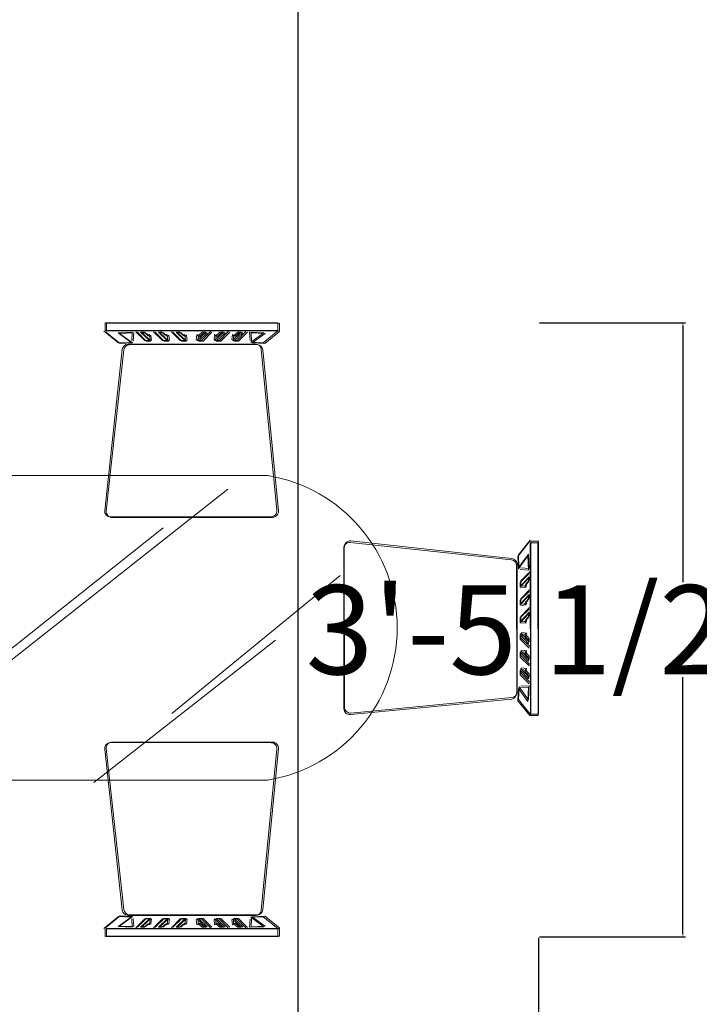
# Model space of a CAD drawing. Units: inches. Extents: x -26 to 575, y -18 to 513.
# Tile 7 of 28: x 77 to 122, y 257 to 324. Entities that reach past the tile are written whole.
import ezdxf

# ---------------------------------------------------------------- set-up
doc = ezdxf.new("R2010")
doc.units = ezdxf.units.IN
doc.header["$MEASUREMENT"] = 0
doc.layers.add('A-ANNO-DIMS', color=2, linetype='Continuous', lineweight=18)
doc.layers.add('Furniture', color=8, linetype='Continuous', lineweight=15)
doc.styles.get("Standard").update_dxf_attribs({"font": 'arial.ttf', "height": 6})
doc.dimstyles.get("Standard").update_dxf_attribs({"dimtxt": 6, "dimasz": 0.18, "dimexe": 0.18, "dimexo": 0.0625, "dimgap": 0.09, "dimtad": 0, "dimtih": 1, "dimtoh": 1, "dimzin": 0, "dimdsep": 46, "dimlunit": 3, "dimtxsty": 'Standard', "dimcen": 0.09, "dimadec": 0, "dimazin": 0, "dimtfac": 1, "dimtofl": 0, "dimtmove": 0, "dimatfit": 3, "dimfxl": 1, "dimtolj": 1, "dimtzin": 0, "dimarcsym": 0})

# ---------------------------------------------------------------- blocks, each defined once
blk = doc.blocks.new('DINING-SET-6-SEAT')
for p, q in [((16.828, 40.76, -3.573), (16.828, 41.278, -3.573)), ((16.828, 41.278, -3.573), (28.461, 41.278, -3.573)), ((16.931, 40.798, -3.573), (16.931, 41.316, -3.573)), ((16.931, 41.316, -3.573), (28.564, 41.316, -3.573)), ((28.461, 41.278, -3.573), (28.461, 40.76, -3.573)), ((28.564, 41.316, -3.573), (28.564, 40.798, -3.573)), ((47.187, 41.329, -3.573), (35.554, 41.319, -3.573)), ((35.554, 41.319, -3.573), (35.554, 40.801, -3.573)), ((47.29, 41.291, -3.573), (35.657, 41.281, -3.573)), ((35.657, 41.281, -3.573), (35.657, 40.763, -3.573)), ((47.188, 40.811, -3.573), (47.187, 41.329, -3.573)), ((47.29, 40.774, -3.573), (47.29, 41.291, -3.573)), ((28.461, 40.76, -3.573), (16.828, 40.76, -3.573)), ((16.828, 40.72, -3.573), (17.824, 39.924, -3.573)), ((28.564, 40.798, -3.573), (16.931, 40.798, -3.573)), ((16.931, 40.758, -3.573), (17.927, 39.962, -3.573)), ((17.784, 40.601, -3.573), (18.74, 40.641, -3.573)), ((18.661, 39.964, -3.573), (17.784, 40.601, -3.573)), ((17.887, 40.639, -3.573), (18.843, 40.679, -3.573)), ((18.763, 40.002, -3.573), (17.887, 40.639, -3.573)), ((18.74, 40.641, -3.573), (18.7, 40.083, -3.573)), ((18.843, 40.679, -3.573), (18.803, 40.121, -3.573)), ((18.979, 40.681, -3.573), (19.577, 40.083, -3.573)), ((19.082, 40.718, -3.573), (19.68, 40.121, -3.573)), ((19.896, 40.083, -3.573), (19.298, 40.641, -3.573)), ((19.298, 40.641, -3.573), (19.537, 40.641, -3.573)), ((19.998, 40.121, -3.573), (19.401, 40.679, -3.573)), ((19.401, 40.679, -3.573), (19.64, 40.679, -3.573)), ((19.537, 40.641, -3.573), (19.816, 40.402, -3.573)), ((19.64, 40.679, -3.573), (19.919, 40.44, -3.573)), ((19.816, 40.402, -3.573), (19.896, 40.481, -3.573)), ((19.896, 40.481, -3.573), (19.936, 40.123, -3.573)), ((19.919, 40.44, -3.573), (19.998, 40.519, -3.573)), ((19.998, 40.519, -3.573), (20.038, 40.161, -3.573)), ((20.175, 40.681, -3.573), (20.772, 40.083, -3.573)), ((20.277, 40.718, -3.573), (20.875, 40.121, -3.573)), ((21.091, 40.083, -3.573), (20.493, 40.641, -3.573)), ((20.493, 40.641, -3.573), (20.732, 40.641, -3.573)), ((21.194, 40.121, -3.573), (20.596, 40.679, -3.573)), ((20.596, 40.679, -3.573), (20.835, 40.679, -3.573)), ((20.732, 40.641, -3.573), (21.011, 40.402, -3.573)), ((20.835, 40.679, -3.573), (21.114, 40.44, -3.573)), ((21.011, 40.402, -3.573), (21.091, 40.481, -3.573)), ((21.091, 40.481, -3.573), (21.131, 40.123, -3.573)), ((21.114, 40.44, -3.573), (21.194, 40.519, -3.573)), ((21.194, 40.519, -3.573), (21.233, 40.161, -3.573)), ((21.37, 40.681, -3.573), (21.967, 40.083, -3.573)), ((21.473, 40.718, -3.573), (22.07, 40.121, -3.573)), ((22.286, 40.083, -3.573), (21.688, 40.641, -3.573)), ((21.688, 40.641, -3.573), (21.928, 40.641, -3.573)), ((22.389, 40.121, -3.573), (21.791, 40.679, -3.573)), ((21.791, 40.679, -3.573), (22.03, 40.679, -3.573)), ((21.928, 40.641, -3.573), (22.206, 40.402, -3.573)), ((22.03, 40.679, -3.573), (22.309, 40.44, -3.573)), ((22.206, 40.402, -3.573), (22.286, 40.481, -3.573)), ((22.286, 40.481, -3.573), (22.326, 40.123, -3.573)), ((22.309, 40.44, -3.573), (22.389, 40.519, -3.573)), ((22.389, 40.519, -3.573), (22.429, 40.161, -3.573)), ((23.083, 40.481, -3.573), (23.043, 40.123, -3.573)), ((23.083, 40.083, -3.573), (23.681, 40.641, -3.573)), ((23.163, 40.402, -3.573), (23.083, 40.481, -3.573)), ((23.186, 40.519, -3.573), (23.146, 40.161, -3.573)), ((23.441, 40.641, -3.573), (23.163, 40.402, -3.573)), ((23.186, 40.121, -3.573), (23.783, 40.679, -3.573)), ((23.265, 40.44, -3.573), (23.186, 40.519, -3.573)), ((23.544, 40.679, -3.573), (23.265, 40.44, -3.573)), ((23.999, 40.681, -3.573), (23.402, 40.083, -3.573)), ((23.681, 40.641, -3.573), (23.441, 40.641, -3.573)), ((24.102, 40.718, -3.573), (23.504, 40.121, -3.573)), ((23.783, 40.679, -3.573), (23.544, 40.679, -3.573)), ((24.278, 40.481, -3.573), (24.238, 40.123, -3.573)), ((24.278, 40.083, -3.573), (24.876, 40.641, -3.573)), ((24.358, 40.402, -3.573), (24.278, 40.481, -3.573)), ((24.381, 40.519, -3.573), (24.341, 40.161, -3.573)), ((24.637, 40.641, -3.573), (24.358, 40.402, -3.573)), ((24.381, 40.121, -3.573), (24.978, 40.679, -3.573)), ((24.461, 40.44, -3.573), (24.381, 40.519, -3.573)), ((24.739, 40.679, -3.573), (24.461, 40.44, -3.573)), ((25.194, 40.681, -3.573), (24.597, 40.083, -3.573)), ((24.876, 40.641, -3.573), (24.637, 40.641, -3.573)), ((25.297, 40.718, -3.573), (24.7, 40.121, -3.573)), ((24.978, 40.679, -3.573), (24.739, 40.679, -3.573)), ((25.473, 40.481, -3.573), (25.434, 40.123, -3.573)), ((25.473, 40.083, -3.573), (26.071, 40.641, -3.573)), ((25.553, 40.402, -3.573), (25.473, 40.481, -3.573)), ((25.576, 40.519, -3.573), (25.536, 40.161, -3.573)), ((25.832, 40.641, -3.573), (25.553, 40.402, -3.573)), ((25.576, 40.121, -3.573), (26.174, 40.679, -3.573)), ((25.656, 40.44, -3.573), (25.576, 40.519, -3.573)), ((25.935, 40.679, -3.573), (25.656, 40.44, -3.573)), ((26.39, 40.681, -3.573), (25.792, 40.083, -3.573)), ((26.071, 40.641, -3.573), (25.832, 40.641, -3.573)), ((26.492, 40.718, -3.573), (25.895, 40.121, -3.573)), ((26.174, 40.679, -3.573), (25.935, 40.679, -3.573)), ((27.585, 40.601, -3.573), (26.629, 40.641, -3.573)), ((26.629, 40.641, -3.573), (26.669, 40.083, -3.573)), ((26.708, 39.964, -3.573), (27.585, 40.601, -3.573)), ((27.688, 40.639, -3.573), (26.731, 40.679, -3.573)), ((26.731, 40.679, -3.573), (26.771, 40.121, -3.573)), ((26.811, 40.002, -3.573), (27.688, 40.639, -3.573)), ((28.541, 40.72, -3.573), (27.545, 39.924, -3.573)), ((28.644, 40.758, -3.573), (27.648, 39.962, -3.573)), ((35.475, 40.761, -3.573), (36.471, 39.966, -3.573)), ((35.554, 40.801, -3.573), (47.188, 40.811, -3.573)), ((35.577, 40.723, -3.573), (36.574, 39.928, -3.573)), ((35.657, 40.763, -3.573), (47.29, 40.774, -3.573)), ((36.431, 40.643, -3.573), (37.387, 40.683, -3.573)), ((37.308, 40.006, -3.573), (36.431, 40.643, -3.573)), ((36.534, 40.605, -3.573), (37.49, 40.646, -3.573)), ((37.411, 39.968, -3.573), (36.534, 40.605, -3.573)), ((37.387, 40.683, -3.573), (37.348, 40.126, -3.573)), ((37.49, 40.646, -3.573), (37.45, 40.088, -3.573)), ((37.626, 40.723, -3.573), (38.224, 40.127, -3.573)), ((37.729, 40.686, -3.573), (38.327, 40.089, -3.573)), ((38.543, 40.127, -3.573), (37.945, 40.684, -3.573)), ((37.945, 40.684, -3.573), (38.184, 40.684, -3.573)), ((38.646, 40.089, -3.573), (38.048, 40.646, -3.573)), ((38.048, 40.646, -3.573), (38.287, 40.646, -3.573)), ((38.184, 40.684, -3.573), (38.463, 40.445, -3.573)), ((38.287, 40.646, -3.573), (38.566, 40.408, -3.573)), ((38.463, 40.445, -3.573), (38.543, 40.525, -3.573)), ((38.543, 40.525, -3.573), (38.583, 40.167, -3.573)), ((38.566, 40.408, -3.573), (38.645, 40.487, -3.573)), ((38.645, 40.487, -3.573), (38.685, 40.129, -3.573)), ((38.821, 40.724, -3.573), (39.419, 40.128, -3.573)), ((38.924, 40.687, -3.573), (39.522, 40.09, -3.573)), ((39.738, 40.128, -3.573), (39.14, 40.685, -3.573)), ((39.14, 40.685, -3.573), (39.379, 40.685, -3.573)), ((39.841, 40.09, -3.573), (39.243, 40.647, -3.573)), ((39.243, 40.647, -3.573), (39.482, 40.647, -3.573)), ((39.379, 40.685, -3.573), (39.658, 40.446, -3.573)), ((39.482, 40.647, -3.573), (39.761, 40.409, -3.573)), ((39.658, 40.446, -3.573), (39.738, 40.526, -3.573)), ((39.738, 40.526, -3.573), (39.778, 40.168, -3.573)), ((39.761, 40.409, -3.573), (39.841, 40.488, -3.573)), ((39.841, 40.488, -3.573), (39.881, 40.13, -3.573)), ((40.016, 40.725, -3.573), (40.615, 40.129, -3.573)), ((40.119, 40.688, -3.573), (40.717, 40.091, -3.573)), ((40.933, 40.129, -3.573), (40.335, 40.686, -3.573)), ((40.335, 40.686, -3.573), (40.574, 40.686, -3.573)), ((41.036, 40.091, -3.573), (40.438, 40.648, -3.573)), ((40.438, 40.648, -3.573), (40.677, 40.648, -3.573)), ((40.574, 40.686, -3.573), (40.853, 40.447, -3.573)), ((40.677, 40.648, -3.573), (40.956, 40.41, -3.573)), ((40.853, 40.447, -3.573), (40.933, 40.527, -3.573)), ((40.933, 40.527, -3.573), (40.973, 40.169, -3.573)), ((40.956, 40.41, -3.573), (41.036, 40.489, -3.573)), ((41.036, 40.489, -3.573), (41.076, 40.131, -3.573)), ((41.73, 40.528, -3.573), (41.69, 40.169, -3.573)), ((41.73, 40.13, -3.573), (42.327, 40.688, -3.573)), ((41.81, 40.448, -3.573), (41.73, 40.528, -3.573)), ((41.833, 40.49, -3.573), (41.793, 40.132, -3.573)), ((42.088, 40.687, -3.573), (41.81, 40.448, -3.573)), ((41.833, 40.092, -3.573), (42.43, 40.65, -3.573)), ((41.912, 40.41, -3.573), (41.833, 40.49, -3.573)), ((42.191, 40.65, -3.573), (41.912, 40.41, -3.573)), ((42.646, 40.728, -3.573), (42.049, 40.13, -3.573)), ((42.327, 40.688, -3.573), (42.088, 40.687, -3.573)), ((42.749, 40.69, -3.573), (42.152, 40.092, -3.573)), ((42.43, 40.65, -3.573), (42.191, 40.65, -3.573)), ((42.925, 40.529, -3.573), (42.885, 40.17, -3.573)), ((42.925, 40.131, -3.573), (43.522, 40.689, -3.573)), ((43.005, 40.449, -3.573), (42.925, 40.529, -3.573)), ((43.028, 40.491, -3.573), (42.988, 40.133, -3.573)), ((43.283, 40.688, -3.573), (43.005, 40.449, -3.573)), ((43.028, 40.093, -3.573), (43.625, 40.651, -3.573)), ((43.108, 40.412, -3.573), (43.028, 40.491, -3.573)), ((43.386, 40.651, -3.573), (43.108, 40.412, -3.573)), ((43.841, 40.729, -3.573), (43.244, 40.131, -3.573)), ((43.522, 40.689, -3.573), (43.283, 40.688, -3.573)), ((43.944, 40.691, -3.573), (43.347, 40.093, -3.573)), ((43.625, 40.651, -3.573), (43.386, 40.651, -3.573)), ((44.12, 40.53, -3.573), (44.081, 40.171, -3.573)), ((44.2, 40.45, -3.573), (44.12, 40.53, -3.573)), ((44.121, 40.132, -3.573), (44.718, 40.69, -3.573)), ((44.223, 40.492, -3.573), (44.183, 40.134, -3.573)), ((44.479, 40.69, -3.573), (44.2, 40.45, -3.573)), ((44.223, 40.094, -3.573), (44.82, 40.652, -3.573)), ((44.303, 40.413, -3.573), (44.223, 40.492, -3.573)), ((44.581, 40.652, -3.573), (44.303, 40.413, -3.573)), ((45.036, 40.73, -3.573), (44.439, 40.132, -3.573)), ((44.718, 40.69, -3.573), (44.479, 40.69, -3.573)), ((45.139, 40.692, -3.573), (44.542, 40.094, -3.573)), ((44.82, 40.652, -3.573), (44.581, 40.652, -3.573)), ((46.232, 40.651, -3.573), (45.275, 40.69, -3.573)), ((45.275, 40.69, -3.573), (45.316, 40.133, -3.573)), ((45.356, 40.013, -3.573), (46.232, 40.651, -3.573)), ((46.334, 40.613, -3.573), (45.378, 40.652, -3.573)), ((45.378, 40.652, -3.573), (45.419, 40.095, -3.573)), ((45.458, 39.976, -3.573), (46.334, 40.613, -3.573)), ((47.188, 40.772, -3.573), (46.192, 39.974, -3.573)), ((47.29, 40.734, -3.573), (46.295, 39.936, -3.573)), ((17.824, 39.924, -3.573), (18.661, 39.964, -3.573)), ((17.927, 39.962, -3.573), (18.763, 40.002, -3.573)), ((26.909, 39.844, -3.573), (18.345, 39.844, -3.573)), ((27.012, 39.882, -3.573), (18.448, 39.882, -3.573)), ((19.577, 40.083, -3.573), (19.896, 40.083, -3.573)), ((19.68, 40.121, -3.573), (19.998, 40.121, -3.573)), ((20.772, 40.083, -3.573), (21.091, 40.083, -3.573)), ((20.875, 40.121, -3.573), (21.194, 40.121, -3.573)), ((21.967, 40.083, -3.573), (22.286, 40.083, -3.573)), ((22.07, 40.121, -3.573), (22.389, 40.121, -3.573)), ((23.402, 40.083, -3.573), (23.083, 40.083, -3.573)), ((23.504, 40.121, -3.573), (23.186, 40.121, -3.573)), ((24.597, 40.083, -3.573), (24.278, 40.083, -3.573)), ((24.7, 40.121, -3.573), (24.381, 40.121, -3.573)), ((25.792, 40.083, -3.573), (25.473, 40.083, -3.573)), ((25.895, 40.121, -3.573), (25.576, 40.121, -3.573)), ((27.545, 39.924, -3.573), (26.708, 39.964, -3.573)), ((27.648, 39.962, -3.573), (26.811, 40.002, -3.573)), ((36.471, 39.966, -3.573), (37.308, 40.006, -3.573)), ((36.574, 39.928, -3.573), (37.411, 39.968, -3.573)), ((37.107, 39.887, -3.573), (45.671, 39.894, -3.573)), ((37.21, 39.849, -3.573), (45.774, 39.856, -3.573)), ((38.224, 40.127, -3.573), (38.543, 40.127, -3.573)), ((38.327, 40.089, -3.573), (38.646, 40.089, -3.573)), ((39.419, 40.128, -3.573), (39.738, 40.128, -3.573)), ((39.522, 40.09, -3.573), (39.841, 40.09, -3.573)), ((40.615, 40.129, -3.573), (40.933, 40.129, -3.573)), ((40.717, 40.091, -3.573), (41.036, 40.091, -3.573)), ((42.049, 40.13, -3.573), (41.73, 40.13, -3.573)), ((42.152, 40.092, -3.573), (41.833, 40.092, -3.573)), ((43.244, 40.131, -3.573), (42.925, 40.131, -3.573)), ((43.347, 40.093, -3.573), (43.028, 40.093, -3.573)), ((44.439, 40.132, -3.573), (44.121, 40.132, -3.573)), ((44.542, 40.094, -3.573), (44.223, 40.094, -3.573)), ((46.192, 39.974, -3.573), (45.356, 40.013, -3.573)), ((46.295, 39.936, -3.573), (45.458, 39.976, -3.573)), ((17.949, 39.484, -3.573), (16.91, 28.653, -3.573)), ((18.052, 39.522, -3.573), (17.012, 28.691, -3.573)), ((28.493, 28.659, -3.573), (27.305, 39.489, -3.573)), ((28.595, 28.696, -3.573), (27.408, 39.527, -3.573)), ((35.534, 28.7, -3.573), (36.712, 39.531, -3.573)), ((35.636, 28.662, -3.573), (36.814, 39.494, -3.573)), ((46.068, 39.534, -3.573), (47.117, 28.704, -3.573)), ((46.171, 39.496, -3.573), (47.219, 28.667, -3.573)), ((16.194, 22.294, -1.308), (26.662, 30.717, -1.308)), ((46.474, 31.041, -1.308), (18.1, 31.041, -1.308)), ((14.74, 19.68, -1.308), (28.116, 30.426, -1.308)), ((25.79, 15.904, -1.308), (43.819, 30.136, -1.308)), ((17.306, 28.217, -3.573), (28.097, 28.217, -3.573)), ((17.409, 28.255, -3.573), (28.199, 28.255, -3.573)), ((46.72, 28.268, -3.573), (35.93, 28.258, -3.573)), ((46.823, 28.23, -3.573), (36.033, 28.22, -3.573)), ((18.1, 10.54, -1.308), (39.457, 27.522, -1.308)), ((0, 14.987, -3.573), (0.01, 26.621, -3.573)), ((0.01, 26.621, -3.573), (0.528, 26.62, -3.573)), ((0.037, 14.884, -3.573), (0.048, 26.518, -3.573)), ((0.048, 26.518, -3.573), (0.565, 26.517, -3.573)), ((0.528, 26.62, -3.573), (0.517, 14.987, -3.573)), ((0.565, 26.517, -3.573), (0.555, 14.884, -3.573)), ((0.567, 26.7, -3.573), (1.363, 25.703, -3.573)), ((0.605, 26.597, -3.573), (1.401, 25.6, -3.573)), ((12.629, 26.641, -3.573), (1.797, 25.463, -3.573)), ((12.667, 26.538, -3.573), (1.835, 25.36, -3.573)), ((52.057, 26.538, -3.573), (62.889, 25.36, -3.573)), ((52.095, 26.641, -3.573), (62.926, 25.463, -3.573)), ((64.119, 26.597, -3.573), (63.323, 25.6, -3.573)), ((64.156, 26.7, -3.573), (63.361, 25.703, -3.573)), ((64.676, 26.518, -3.573), (64.159, 26.517, -3.573)), ((64.159, 26.517, -3.573), (64.169, 14.884, -3.573)), ((64.714, 26.621, -3.573), (64.196, 26.62, -3.573)), ((64.196, 26.62, -3.573), (64.207, 14.987, -3.573)), ((64.686, 14.884, -3.573), (64.676, 26.518, -3.573)), ((64.724, 14.987, -3.573), (64.714, 26.621, -3.573)), ((13.061, 15.454, -3.573), (13.071, 26.244, -3.573)), ((13.099, 15.351, -3.573), (13.108, 26.142, -3.573)), ((51.625, 15.351, -3.573), (51.615, 26.142, -3.573)), ((51.663, 15.454, -3.573), (51.653, 26.244, -3.573)), ((0.686, 25.744, -3.573), (0.645, 24.787, -3.573)), ((0.724, 25.641, -3.573), (0.683, 24.685, -3.573)), ((1.322, 24.866, -3.573), (0.686, 25.744, -3.573)), ((1.36, 24.764, -3.573), (0.724, 25.641, -3.573)), ((1.363, 25.703, -3.573), (1.322, 24.866, -3.573)), ((1.401, 25.6, -3.573), (1.36, 24.764, -3.573)), ((63.323, 25.6, -3.573), (63.364, 24.764, -3.573)), ((63.361, 25.703, -3.573), (63.401, 24.866, -3.573)), ((63.364, 24.764, -3.573), (64, 25.641, -3.573)), ((63.401, 24.866, -3.573), (64.038, 25.744, -3.573)), ((64, 25.641, -3.573), (64.041, 24.685, -3.573)), ((64.038, 25.744, -3.573), (64.078, 24.787, -3.573)), ((0.605, 24.548, -3.573), (1.202, 23.95, -3.573)), ((0.645, 24.787, -3.573), (1.203, 24.827, -3.573)), ((0.683, 24.685, -3.573), (1.241, 24.724, -3.573)), ((1.442, 25.067, -3.573), (1.435, 16.503, -3.573)), ((1.48, 24.964, -3.573), (1.472, 16.401, -3.573)), ((63.244, 24.964, -3.573), (63.252, 16.401, -3.573)), ((63.282, 25.067, -3.573), (63.289, 16.503, -3.573)), ((64.041, 24.685, -3.573), (63.483, 24.724, -3.573)), ((64.078, 24.787, -3.573), (63.521, 24.827, -3.573)), ((64.118, 24.548, -3.573), (63.522, 23.95, -3.573)), ((0.643, 24.446, -3.573), (1.24, 23.847, -3.573)), ((1.202, 23.632, -3.573), (0.645, 24.23, -3.573)), ((0.645, 24.23, -3.573), (0.645, 23.991, -3.573)), ((0.645, 23.991, -3.573), (0.883, 23.712, -3.573)), ((0.683, 24.127, -3.573), (0.682, 23.888, -3.573)), ((0.682, 23.888, -3.573), (0.921, 23.609, -3.573)), ((1.24, 23.529, -3.573), (0.683, 24.127, -3.573)), ((1.202, 23.95, -3.573), (1.202, 23.632, -3.573)), ((40.039, 15.033, -1.308), (51.38, 24.327, -1.308)), ((64.081, 24.446, -3.573), (63.484, 23.847, -3.573)), ((63.484, 23.529, -3.573), (64.041, 24.127, -3.573)), ((63.522, 23.632, -3.573), (64.079, 24.23, -3.573)), ((63.522, 23.95, -3.573), (63.522, 23.632, -3.573)), ((64.041, 23.888, -3.573), (63.803, 23.609, -3.573)), ((64.079, 23.991, -3.573), (63.84, 23.712, -3.573)), ((64.041, 24.127, -3.573), (64.041, 23.888, -3.573)), ((64.079, 24.23, -3.573), (64.079, 23.991, -3.573)), ((0.604, 23.353, -3.573), (1.201, 22.755, -3.573)), ((0.642, 23.25, -3.573), (1.239, 22.652, -3.573)), ((0.883, 23.712, -3.573), (0.804, 23.632, -3.573)), ((0.804, 23.632, -3.573), (1.162, 23.592, -3.573)), ((0.921, 23.609, -3.573), (0.841, 23.529, -3.573)), ((0.841, 23.529, -3.573), (1.2, 23.489, -3.573)), ((1.24, 23.847, -3.573), (1.24, 23.529, -3.573)), ((63.484, 23.847, -3.573), (63.484, 23.529, -3.573)), ((64.082, 23.25, -3.573), (63.485, 22.652, -3.573)), ((64.12, 23.353, -3.573), (63.523, 22.755, -3.573)), ((63.882, 23.529, -3.573), (63.524, 23.489, -3.573)), ((63.92, 23.632, -3.573), (63.562, 23.592, -3.573)), ((63.803, 23.609, -3.573), (63.882, 23.529, -3.573)), ((63.84, 23.712, -3.573), (63.92, 23.632, -3.573)), ((1.201, 22.436, -3.573), (0.644, 23.034, -3.573)), ((0.644, 23.034, -3.573), (0.644, 22.795, -3.573)), ((0.644, 22.795, -3.573), (0.882, 22.516, -3.573)), ((0.682, 22.932, -3.573), (0.681, 22.693, -3.573)), ((0.681, 22.693, -3.573), (0.92, 22.414, -3.573)), ((1.239, 22.334, -3.573), (0.682, 22.932, -3.573)), ((1.201, 22.755, -3.573), (1.201, 22.436, -3.573)), ((1.239, 22.652, -3.573), (1.239, 22.334, -3.573)), ((63.485, 22.334, -3.573), (64.042, 22.932, -3.573)), ((63.485, 22.652, -3.573), (63.485, 22.334, -3.573)), ((63.523, 22.436, -3.573), (64.08, 23.034, -3.573)), ((63.523, 22.755, -3.573), (63.523, 22.436, -3.573)), ((64.042, 22.693, -3.573), (63.804, 22.414, -3.573)), ((64.08, 22.795, -3.573), (63.842, 22.516, -3.573)), ((64.042, 22.932, -3.573), (64.042, 22.693, -3.573)), ((64.08, 23.034, -3.573), (64.08, 22.795, -3.573)), ((0.603, 22.158, -3.573), (1.2, 21.56, -3.573)), ((0.641, 22.055, -3.573), (1.238, 21.457, -3.573)), ((0.882, 22.516, -3.573), (0.803, 22.437, -3.573)), ((0.803, 22.437, -3.573), (1.161, 22.397, -3.573)), ((0.92, 22.414, -3.573), (0.84, 22.334, -3.573)), ((0.84, 22.334, -3.573), (1.199, 22.294, -3.573)), ((64.083, 22.055, -3.573), (63.486, 21.457, -3.573)), ((64.121, 22.158, -3.573), (63.524, 21.56, -3.573)), ((63.883, 22.334, -3.573), (63.525, 22.294, -3.573)), ((63.921, 22.437, -3.573), (63.563, 22.397, -3.573)), ((63.804, 22.414, -3.573), (63.883, 22.334, -3.573)), ((63.842, 22.516, -3.573), (63.921, 22.437, -3.573)), ((1.2, 21.241, -3.573), (0.643, 21.839, -3.573)), ((0.643, 21.839, -3.573), (0.643, 21.6, -3.573)), ((0.643, 21.6, -3.573), (0.881, 21.321, -3.573)), ((0.681, 21.736, -3.573), (0.68, 21.497, -3.573)), ((0.68, 21.497, -3.573), (0.919, 21.218, -3.573)), ((1.238, 21.138, -3.573), (0.681, 21.736, -3.573)), ((0.881, 21.321, -3.573), (0.802, 21.241, -3.573)), ((0.802, 21.241, -3.573), (1.16, 21.201, -3.573)), ((0.919, 21.218, -3.573), (0.839, 21.139, -3.573)), ((1.2, 21.56, -3.573), (1.2, 21.241, -3.573)), ((1.238, 21.457, -3.573), (1.238, 21.138, -3.573)), ((63.486, 21.138, -3.573), (64.043, 21.736, -3.573)), ((63.486, 21.457, -3.573), (63.486, 21.138, -3.573)), ((63.524, 21.241, -3.573), (64.081, 21.839, -3.573)), ((63.524, 21.56, -3.573), (63.524, 21.241, -3.573)), ((63.922, 21.241, -3.573), (63.564, 21.201, -3.573)), ((64.043, 21.497, -3.573), (63.805, 21.218, -3.573)), ((63.805, 21.218, -3.573), (63.884, 21.139, -3.573)), ((64.081, 21.6, -3.573), (63.843, 21.321, -3.573)), ((63.843, 21.321, -3.573), (63.922, 21.241, -3.573)), ((64.043, 21.736, -3.573), (64.043, 21.497, -3.573)), ((64.081, 21.839, -3.573), (64.081, 21.6, -3.573)), ((0.839, 21.139, -3.573), (1.198, 21.099, -3.573)), ((63.884, 21.139, -3.573), (63.526, 21.099, -3.573)), ((0.601, 19.529, -3.573), (1.199, 20.126, -3.573)), ((0.639, 19.426, -3.573), (1.237, 20.023, -3.573)), ((1.199, 20.444, -3.573), (0.641, 19.847, -3.573)), ((0.641, 20.086, -3.573), (0.88, 20.365, -3.573)), ((0.641, 19.847, -3.573), (0.641, 20.086, -3.573)), ((1.237, 20.342, -3.573), (0.679, 19.744, -3.573)), ((0.679, 19.983, -3.573), (0.918, 20.262, -3.573)), ((0.679, 19.744, -3.573), (0.679, 19.983, -3.573)), ((0.801, 20.445, -3.573), (1.159, 20.484, -3.573)), ((0.88, 20.365, -3.573), (0.801, 20.445, -3.573)), ((0.839, 20.342, -3.573), (1.197, 20.381, -3.573)), ((0.918, 20.262, -3.573), (0.839, 20.342, -3.573)), ((1.199, 20.126, -3.573), (1.199, 20.444, -3.573)), ((1.237, 20.023, -3.573), (1.237, 20.342, -3.573)), ((34.805, 10.386, -1.308), (47.018, 19.971, -1.308)), ((63.487, 20.023, -3.573), (63.487, 20.342, -3.573)), ((63.487, 20.342, -3.573), (64.045, 19.744, -3.573)), ((64.085, 19.426, -3.573), (63.487, 20.023, -3.573)), ((63.525, 20.126, -3.573), (63.525, 20.444, -3.573)), ((63.525, 20.444, -3.573), (64.083, 19.847, -3.573)), ((64.123, 19.529, -3.573), (63.525, 20.126, -3.573)), ((63.885, 20.342, -3.573), (63.527, 20.381, -3.573)), ((63.923, 20.445, -3.573), (63.565, 20.484, -3.573)), ((63.806, 20.262, -3.573), (63.885, 20.342, -3.573)), ((64.045, 19.983, -3.573), (63.806, 20.262, -3.573)), ((63.843, 20.365, -3.573), (63.923, 20.445, -3.573)), ((64.083, 20.086, -3.573), (63.843, 20.365, -3.573)), ((64.045, 19.744, -3.573), (64.045, 19.983, -3.573)), ((64.083, 19.847, -3.573), (64.083, 20.086, -3.573)), ((1.198, 19.249, -3.573), (0.64, 18.652, -3.573)), ((0.8, 19.249, -3.573), (1.158, 19.289, -3.573)), ((0.879, 19.17, -3.573), (0.8, 19.249, -3.573)), ((1.198, 18.93, -3.573), (1.198, 19.249, -3.573)), ((63.526, 18.93, -3.573), (63.526, 19.249, -3.573)), ((63.526, 19.249, -3.573), (64.084, 18.652, -3.573)), ((63.924, 19.249, -3.573), (63.566, 19.289, -3.573)), ((63.844, 19.17, -3.573), (63.924, 19.249, -3.573)), ((0.6, 18.333, -3.573), (1.198, 18.93, -3.573)), ((0.638, 18.231, -3.573), (1.236, 18.828, -3.573)), ((0.64, 18.891, -3.573), (0.879, 19.17, -3.573)), ((0.64, 18.652, -3.573), (0.64, 18.891, -3.573)), ((1.236, 19.146, -3.573), (0.678, 18.549, -3.573)), ((0.678, 18.788, -3.573), (0.917, 19.067, -3.573)), ((0.678, 18.549, -3.573), (0.678, 18.788, -3.573)), ((0.838, 19.147, -3.573), (1.196, 19.186, -3.573)), ((0.917, 19.067, -3.573), (0.838, 19.147, -3.573)), ((1.236, 18.828, -3.573), (1.236, 19.146, -3.573)), ((63.488, 18.828, -3.573), (63.488, 19.146, -3.573)), ((63.488, 19.146, -3.573), (64.046, 18.549, -3.573)), ((64.086, 18.231, -3.573), (63.488, 18.828, -3.573)), ((64.124, 18.333, -3.573), (63.526, 18.93, -3.573)), ((63.886, 19.147, -3.573), (63.528, 19.186, -3.573)), ((63.807, 19.067, -3.573), (63.886, 19.147, -3.573)), ((64.046, 18.788, -3.573), (63.807, 19.067, -3.573)), ((64.084, 18.891, -3.573), (63.844, 19.17, -3.573)), ((64.046, 18.549, -3.573), (64.046, 18.788, -3.573)), ((64.084, 18.652, -3.573), (64.084, 18.891, -3.573)), ((1.197, 18.054, -3.573), (0.639, 17.457, -3.573)), ((0.639, 17.696, -3.573), (0.878, 17.974, -3.573)), ((1.235, 17.951, -3.573), (0.677, 17.354, -3.573)), ((0.799, 18.054, -3.573), (1.157, 18.094, -3.573)), ((0.878, 17.974, -3.573), (0.799, 18.054, -3.573)), ((0.837, 17.951, -3.573), (1.195, 17.991, -3.573)), ((0.916, 17.872, -3.573), (0.837, 17.951, -3.573)), ((1.197, 17.735, -3.573), (1.197, 18.054, -3.573)), ((1.234, 17.632, -3.573), (1.235, 17.951, -3.573)), ((63.489, 17.632, -3.573), (63.489, 17.951, -3.573)), ((63.489, 17.951, -3.573), (64.047, 17.354, -3.573)), ((63.527, 17.735, -3.573), (63.527, 18.054, -3.573)), ((63.527, 18.054, -3.573), (64.085, 17.457, -3.573)), ((63.887, 17.951, -3.573), (63.529, 17.991, -3.573)), ((63.925, 18.054, -3.573), (63.567, 18.094, -3.573)), ((63.808, 17.872, -3.573), (63.887, 17.951, -3.573)), ((63.846, 17.974, -3.573), (63.925, 18.054, -3.573)), ((64.085, 17.696, -3.573), (63.846, 17.974, -3.573)), ((0.599, 17.138, -3.573), (1.197, 17.735, -3.573)), ((0.637, 17.035, -3.573), (1.234, 17.632, -3.573)), ((0.639, 17.457, -3.573), (0.639, 17.696, -3.573)), ((0.677, 17.593, -3.573), (0.916, 17.872, -3.573)), ((0.677, 17.354, -3.573), (0.677, 17.593, -3.573)), ((64.087, 17.035, -3.573), (63.489, 17.632, -3.573)), ((64.125, 17.138, -3.573), (63.527, 17.735, -3.573)), ((64.047, 17.593, -3.573), (63.808, 17.872, -3.573)), ((64.047, 17.354, -3.573), (64.047, 17.593, -3.573)), ((64.085, 17.457, -3.573), (64.085, 17.696, -3.573)), ((0.677, 15.943, -3.573), (0.639, 16.899, -3.573)), ((0.639, 16.899, -3.573), (1.196, 16.859, -3.573)), ((0.715, 15.84, -3.573), (0.676, 16.796, -3.573)), ((0.676, 16.796, -3.573), (1.234, 16.756, -3.573)), ((1.315, 16.819, -3.573), (0.677, 15.943, -3.573)), ((1.353, 16.716, -3.573), (0.715, 15.84, -3.573)), ((1.354, 15.982, -3.573), (1.315, 16.819, -3.573)), ((1.392, 15.879, -3.573), (1.353, 16.716, -3.573)), ((63.332, 15.879, -3.573), (63.371, 16.716, -3.573)), ((63.369, 15.982, -3.573), (63.408, 16.819, -3.573)), ((63.371, 16.716, -3.573), (64.009, 15.84, -3.573)), ((63.408, 16.819, -3.573), (64.046, 15.943, -3.573)), ((64.048, 16.796, -3.573), (63.49, 16.756, -3.573)), ((64.085, 16.899, -3.573), (63.528, 16.859, -3.573)), ((64.009, 15.84, -3.573), (64.048, 16.796, -3.573)), ((64.046, 15.943, -3.573), (64.085, 16.899, -3.573)), ((0.557, 14.987, -3.573), (1.354, 15.982, -3.573)), ((1.795, 16.106, -3.573), (12.624, 15.058, -3.573)), ((1.832, 16.004, -3.573), (12.662, 14.955, -3.573)), ((62.892, 16.004, -3.573), (52.062, 14.955, -3.573)), ((62.929, 16.106, -3.573), (52.099, 15.058, -3.573)), ((64.167, 14.987, -3.573), (63.369, 15.982, -3.573)), ((0.595, 14.884, -3.573), (1.392, 15.879, -3.573)), ((64.129, 14.884, -3.573), (63.332, 15.879, -3.573)), ((0.517, 14.987, -3.573), (0, 14.987, -3.573)), ((0.555, 14.884, -3.573), (0.037, 14.884, -3.573)), ((64.169, 14.884, -3.573), (64.686, 14.884, -3.573)), ((64.207, 14.987, -3.573), (64.724, 14.987, -3.573)), ((17.949, 1.845, -3.573), (16.91, 12.676, -3.573)), ((18.052, 1.807, -3.573), (17.012, 12.638, -3.573)), ((17.306, 13.113, -3.573), (28.097, 13.113, -3.573)), ((17.409, 13.075, -3.573), (28.199, 13.075, -3.573)), ((28.493, 12.671, -3.573), (27.305, 1.84, -3.573)), ((28.595, 12.633, -3.573), (27.408, 1.802, -3.573)), ((35.534, 12.63, -3.573), (36.712, 1.798, -3.573)), ((35.636, 12.668, -3.573), (36.814, 1.836, -3.573)), ((46.72, 13.062, -3.573), (35.93, 13.071, -3.573)), ((46.823, 13.1, -3.573), (36.033, 13.109, -3.573)), ((46.068, 1.795, -3.573), (47.117, 12.625, -3.573)), ((46.171, 1.833, -3.573), (47.219, 12.663, -3.573)), ((18.1, 10.54, -1.308), (46.474, 10.54, -1.308)), ((16.828, 0.609, -3.573), (17.824, 1.405, -3.573)), ((16.931, 0.571, -3.573), (17.927, 1.367, -3.573)), ((18.661, 1.366, -3.573), (17.784, 0.728, -3.573)), ((17.824, 1.405, -3.573), (18.661, 1.366, -3.573)), ((18.763, 1.328, -3.573), (17.887, 0.691, -3.573)), ((17.927, 1.367, -3.573), (18.763, 1.328, -3.573)), ((26.909, 1.485, -3.573), (18.345, 1.485, -3.573)), ((27.012, 1.447, -3.573), (18.448, 1.447, -3.573)), ((27.545, 1.405, -3.573), (26.708, 1.366, -3.573)), ((26.708, 1.366, -3.573), (27.585, 0.728, -3.573)), ((27.648, 1.367, -3.573), (26.811, 1.328, -3.573)), ((26.811, 1.328, -3.573), (27.688, 0.691, -3.573)), ((28.541, 0.609, -3.573), (27.545, 1.405, -3.573)), ((28.644, 0.571, -3.573), (27.648, 1.367, -3.573)), ((35.475, 0.568, -3.573), (36.471, 1.364, -3.573)), ((35.577, 0.606, -3.573), (36.574, 1.401, -3.573)), ((36.471, 1.364, -3.573), (37.308, 1.323, -3.573)), ((37.411, 1.361, -3.573), (36.534, 0.724, -3.573)), ((36.574, 1.401, -3.573), (37.411, 1.361, -3.573)), ((37.107, 1.443, -3.573), (45.671, 1.435, -3.573)), ((37.21, 1.48, -3.573), (45.774, 1.473, -3.573)), ((46.192, 1.355, -3.573), (45.356, 1.316, -3.573)), ((46.295, 1.393, -3.573), (45.458, 1.354, -3.573)), ((45.458, 1.354, -3.573), (46.334, 0.716, -3.573)), ((47.188, 0.558, -3.573), (46.192, 1.355, -3.573)), ((47.29, 0.596, -3.573), (46.295, 1.393, -3.573)), ((17.784, 0.728, -3.573), (18.74, 0.689, -3.573)), ((17.887, 0.691, -3.573), (18.843, 0.651, -3.573)), ((18.74, 0.689, -3.573), (18.7, 1.246, -3.573)), ((18.843, 0.651, -3.573), (18.803, 1.208, -3.573)), ((18.979, 0.649, -3.573), (19.577, 1.246, -3.573)), ((19.082, 0.611, -3.573), (19.68, 1.208, -3.573)), ((19.896, 1.246, -3.573), (19.298, 0.689, -3.573)), ((19.298, 0.689, -3.573), (19.537, 0.689, -3.573)), ((19.998, 1.208, -3.573), (19.401, 0.651, -3.573)), ((19.537, 0.689, -3.573), (19.816, 0.928, -3.573)), ((19.577, 1.246, -3.573), (19.896, 1.246, -3.573)), ((19.64, 0.651, -3.573), (19.919, 0.89, -3.573)), ((19.68, 1.208, -3.573), (19.998, 1.208, -3.573)), ((19.816, 0.928, -3.573), (19.896, 0.848, -3.573)), ((19.896, 0.848, -3.573), (19.936, 1.206, -3.573)), ((19.919, 0.89, -3.573), (19.998, 0.81, -3.573)), ((19.998, 0.81, -3.573), (20.038, 1.168, -3.573)), ((20.175, 0.649, -3.573), (20.772, 1.246, -3.573)), ((20.277, 0.611, -3.573), (20.875, 1.208, -3.573)), ((21.091, 1.246, -3.573), (20.493, 0.689, -3.573)), ((20.493, 0.689, -3.573), (20.732, 0.689, -3.573)), ((21.194, 1.208, -3.573), (20.596, 0.651, -3.573)), ((20.732, 0.689, -3.573), (21.011, 0.928, -3.573)), ((20.772, 1.246, -3.573), (21.091, 1.246, -3.573)), ((20.835, 0.651, -3.573), (21.114, 0.89, -3.573)), ((20.875, 1.208, -3.573), (21.194, 1.208, -3.573)), ((21.011, 0.928, -3.573), (21.091, 0.848, -3.573)), ((21.091, 0.848, -3.573), (21.131, 1.206, -3.573)), ((21.114, 0.89, -3.573), (21.194, 0.81, -3.573)), ((21.194, 0.81, -3.573), (21.233, 1.168, -3.573)), ((21.37, 0.649, -3.573), (21.967, 1.246, -3.573)), ((21.473, 0.611, -3.573), (22.07, 1.208, -3.573)), ((22.286, 1.246, -3.573), (21.688, 0.689, -3.573)), ((21.688, 0.689, -3.573), (21.928, 0.689, -3.573)), ((22.389, 1.208, -3.573), (21.791, 0.651, -3.573)), ((21.928, 0.689, -3.573), (22.206, 0.928, -3.573)), ((21.967, 1.246, -3.573), (22.286, 1.246, -3.573)), ((22.03, 0.651, -3.573), (22.309, 0.89, -3.573)), ((22.07, 1.208, -3.573), (22.389, 1.208, -3.573)), ((22.206, 0.928, -3.573), (22.286, 0.848, -3.573)), ((22.286, 0.848, -3.573), (22.326, 1.206, -3.573)), ((22.309, 0.89, -3.573), (22.389, 0.81, -3.573)), ((22.389, 0.81, -3.573), (22.429, 1.168, -3.573)), ((23.083, 0.848, -3.573), (23.043, 1.206, -3.573)), ((23.402, 1.246, -3.573), (23.083, 1.246, -3.573)), ((23.083, 1.246, -3.573), (23.681, 0.689, -3.573)), ((23.163, 0.928, -3.573), (23.083, 0.848, -3.573)), ((23.186, 0.81, -3.573), (23.146, 1.168, -3.573)), ((23.441, 0.689, -3.573), (23.163, 0.928, -3.573)), ((23.504, 1.208, -3.573), (23.186, 1.208, -3.573)), ((23.186, 1.208, -3.573), (23.783, 0.651, -3.573)), ((23.265, 0.89, -3.573), (23.186, 0.81, -3.573)), ((23.544, 0.651, -3.573), (23.265, 0.89, -3.573)), ((23.999, 0.649, -3.573), (23.402, 1.246, -3.573)), ((23.681, 0.689, -3.573), (23.441, 0.689, -3.573)), ((24.102, 0.611, -3.573), (23.504, 1.208, -3.573)), ((24.278, 0.848, -3.573), (24.238, 1.206, -3.573)), ((24.597, 1.246, -3.573), (24.278, 1.246, -3.573)), ((24.278, 1.246, -3.573), (24.876, 0.689, -3.573)), ((24.358, 0.928, -3.573), (24.278, 0.848, -3.573)), ((24.381, 0.81, -3.573), (24.341, 1.168, -3.573)), ((24.637, 0.689, -3.573), (24.358, 0.928, -3.573)), ((24.7, 1.208, -3.573), (24.381, 1.208, -3.573)), ((24.381, 1.208, -3.573), (24.978, 0.651, -3.573)), ((24.461, 0.89, -3.573), (24.381, 0.81, -3.573)), ((24.739, 0.651, -3.573), (24.461, 0.89, -3.573)), ((25.194, 0.649, -3.573), (24.597, 1.246, -3.573)), ((24.876, 0.689, -3.573), (24.637, 0.689, -3.573)), ((25.297, 0.611, -3.573), (24.7, 1.208, -3.573)), ((25.473, 0.848, -3.573), (25.434, 1.206, -3.573)), ((25.792, 1.246, -3.573), (25.473, 1.246, -3.573)), ((25.473, 1.246, -3.573), (26.071, 0.689, -3.573)), ((25.553, 0.928, -3.573), (25.473, 0.848, -3.573)), ((25.576, 0.81, -3.573), (25.536, 1.168, -3.573)), ((25.832, 0.689, -3.573), (25.553, 0.928, -3.573)), ((25.895, 1.208, -3.573), (25.576, 1.208, -3.573)), ((25.576, 1.208, -3.573), (26.174, 0.651, -3.573)), ((25.656, 0.89, -3.573), (25.576, 0.81, -3.573)), ((25.935, 0.651, -3.573), (25.656, 0.89, -3.573)), ((26.39, 0.649, -3.573), (25.792, 1.246, -3.573)), ((26.071, 0.689, -3.573), (25.832, 0.689, -3.573)), ((26.492, 0.611, -3.573), (25.895, 1.208, -3.573)), ((26.629, 0.689, -3.573), (26.669, 1.246, -3.573)), ((27.585, 0.728, -3.573), (26.629, 0.689, -3.573)), ((26.731, 0.651, -3.573), (26.771, 1.208, -3.573)), ((27.688, 0.691, -3.573), (26.731, 0.651, -3.573)), ((37.308, 1.323, -3.573), (36.431, 0.687, -3.573)), ((36.431, 0.687, -3.573), (37.387, 0.646, -3.573)), ((36.534, 0.724, -3.573), (37.49, 0.684, -3.573)), ((37.387, 0.646, -3.573), (37.348, 1.204, -3.573)), ((37.49, 0.684, -3.573), (37.45, 1.241, -3.573)), ((37.626, 0.606, -3.573), (38.224, 1.203, -3.573)), ((37.729, 0.644, -3.573), (38.327, 1.241, -3.573)), ((38.543, 1.203, -3.573), (37.945, 0.646, -3.573)), ((38.646, 1.24, -3.573), (38.048, 0.683, -3.573)), ((38.048, 0.683, -3.573), (38.287, 0.683, -3.573)), ((38.184, 0.645, -3.573), (38.463, 0.884, -3.573)), ((38.224, 1.203, -3.573), (38.543, 1.203, -3.573)), ((38.287, 0.683, -3.573), (38.566, 0.922, -3.573)), ((38.327, 1.241, -3.573), (38.646, 1.24, -3.573)), ((38.463, 0.884, -3.573), (38.543, 0.804, -3.573)), ((38.543, 0.804, -3.573), (38.583, 1.163, -3.573)), ((38.566, 0.922, -3.573), (38.645, 0.842, -3.573)), ((38.645, 0.842, -3.573), (38.685, 1.2, -3.573)), ((38.821, 0.605, -3.573), (39.419, 1.202, -3.573)), ((38.924, 0.643, -3.573), (39.522, 1.24, -3.573)), ((39.738, 1.201, -3.573), (39.14, 0.645, -3.573)), ((39.841, 1.239, -3.573), (39.243, 0.682, -3.573)), ((39.243, 0.682, -3.573), (39.482, 0.682, -3.573)), ((39.379, 0.644, -3.573), (39.658, 0.883, -3.573)), ((39.419, 1.202, -3.573), (39.738, 1.201, -3.573)), ((39.482, 0.682, -3.573), (39.761, 0.921, -3.573)), ((39.522, 1.24, -3.573), (39.841, 1.239, -3.573)), ((39.658, 0.883, -3.573), (39.738, 0.803, -3.573)), ((39.738, 0.803, -3.573), (39.778, 1.162, -3.573)), ((39.761, 0.921, -3.573), (39.841, 0.841, -3.573)), ((39.841, 0.841, -3.573), (39.881, 1.199, -3.573)), ((40.016, 0.604, -3.573), (40.615, 1.201, -3.573)), ((40.119, 0.642, -3.573), (40.717, 1.238, -3.573)), ((40.933, 1.2, -3.573), (40.335, 0.643, -3.573)), ((41.036, 1.238, -3.573), (40.438, 0.681, -3.573)), ((40.438, 0.681, -3.573), (40.677, 0.681, -3.573)), ((40.574, 0.643, -3.573), (40.853, 0.882, -3.573)), ((40.615, 1.201, -3.573), (40.933, 1.2, -3.573)), ((40.677, 0.681, -3.573), (40.956, 0.92, -3.573)), ((40.717, 1.238, -3.573), (41.036, 1.238, -3.573)), ((40.853, 0.882, -3.573), (40.933, 0.802, -3.573)), ((40.933, 0.802, -3.573), (40.973, 1.161, -3.573)), ((40.956, 0.92, -3.573), (41.036, 0.84, -3.573)), ((41.036, 0.84, -3.573), (41.076, 1.198, -3.573)), ((41.73, 0.802, -3.573), (41.69, 1.16, -3.573)), ((42.049, 1.199, -3.573), (41.73, 1.2, -3.573)), ((41.73, 1.2, -3.573), (42.327, 0.642, -3.573)), ((41.81, 0.881, -3.573), (41.73, 0.802, -3.573)), ((41.833, 0.839, -3.573), (41.793, 1.198, -3.573)), ((42.088, 0.642, -3.573), (41.81, 0.881, -3.573)), ((42.152, 1.237, -3.573), (41.833, 1.238, -3.573)), ((41.833, 1.238, -3.573), (42.43, 0.679, -3.573)), ((41.912, 0.919, -3.573), (41.833, 0.839, -3.573)), ((42.191, 0.68, -3.573), (41.912, 0.919, -3.573)), ((42.646, 0.602, -3.573), (42.049, 1.199, -3.573)), ((42.749, 0.639, -3.573), (42.152, 1.237, -3.573)), ((42.43, 0.679, -3.573), (42.191, 0.68, -3.573)), ((42.925, 0.8, -3.573), (42.885, 1.159, -3.573)), ((43.244, 1.198, -3.573), (42.925, 1.199, -3.573)), ((42.925, 1.199, -3.573), (43.522, 0.641, -3.573)), ((43.005, 0.88, -3.573), (42.925, 0.8, -3.573)), ((43.028, 0.838, -3.573), (42.988, 1.197, -3.573)), ((43.283, 0.641, -3.573), (43.005, 0.88, -3.573)), ((43.347, 1.236, -3.573), (43.028, 1.236, -3.573)), ((43.028, 1.236, -3.573), (43.625, 0.678, -3.573)), ((43.108, 0.918, -3.573), (43.028, 0.838, -3.573)), ((43.386, 0.679, -3.573), (43.108, 0.918, -3.573)), ((43.841, 0.601, -3.573), (43.244, 1.198, -3.573)), ((43.944, 0.638, -3.573), (43.347, 1.236, -3.573)), ((43.625, 0.678, -3.573), (43.386, 0.679, -3.573)), ((44.12, 0.799, -3.573), (44.081, 1.158, -3.573)), ((44.2, 0.879, -3.573), (44.12, 0.799, -3.573)), ((44.439, 1.197, -3.573), (44.121, 1.198, -3.573)), ((44.121, 1.198, -3.573), (44.718, 0.64, -3.573)), ((44.223, 0.837, -3.573), (44.183, 1.196, -3.573)), ((44.479, 0.64, -3.573), (44.2, 0.879, -3.573)), ((44.542, 1.235, -3.573), (44.223, 1.235, -3.573)), ((44.223, 1.235, -3.573), (44.82, 0.677, -3.573)), ((44.303, 0.917, -3.573), (44.223, 0.837, -3.573)), ((44.581, 0.678, -3.573), (44.303, 0.917, -3.573)), ((45.036, 0.6, -3.573), (44.439, 1.197, -3.573)), ((45.139, 0.637, -3.573), (44.542, 1.235, -3.573)), ((44.82, 0.677, -3.573), (44.581, 0.678, -3.573)), ((45.275, 0.639, -3.573), (45.316, 1.197, -3.573)), ((46.232, 0.678, -3.573), (45.275, 0.639, -3.573)), ((45.356, 1.316, -3.573), (46.232, 0.678, -3.573)), ((45.378, 0.677, -3.573), (45.419, 1.234, -3.573)), ((46.334, 0.716, -3.573), (45.378, 0.677, -3.573)), ((28.461, 0.569, -3.573), (16.828, 0.569, -3.573)), ((16.828, 0.569, -3.573), (16.828, 0.051, -3.573)), ((16.828, 0.051, -3.573), (28.461, 0.051, -3.573)), ((28.564, 0.531, -3.573), (16.931, 0.531, -3.573)), ((16.931, 0.531, -3.573), (16.931, 0.014, -3.573)), ((16.931, 0.014, -3.573), (28.564, 0.014, -3.573)), ((19.401, 0.651, -3.573), (19.64, 0.651, -3.573)), ((20.596, 0.651, -3.573), (20.835, 0.651, -3.573)), ((21.791, 0.651, -3.573), (22.03, 0.651, -3.573)), ((23.783, 0.651, -3.573), (23.544, 0.651, -3.573)), ((24.978, 0.651, -3.573), (24.739, 0.651, -3.573)), ((26.174, 0.651, -3.573), (25.935, 0.651, -3.573)), ((28.461, 0.051, -3.573), (28.461, 0.569, -3.573)), ((28.564, 0.014, -3.573), (28.564, 0.531, -3.573)), ((35.554, 0.011, -3.573), (35.554, 0.528, -3.573)), ((35.554, 0.528, -3.573), (47.188, 0.518, -3.573)), ((47.187, 0, -3.573), (35.554, 0.011, -3.573)), ((35.657, 0.048, -3.573), (35.657, 0.566, -3.573)), ((35.657, 0.566, -3.573), (47.29, 0.556, -3.573)), ((47.29, 0.038, -3.573), (35.657, 0.048, -3.573)), ((37.945, 0.646, -3.573), (38.184, 0.645, -3.573)), ((39.14, 0.645, -3.573), (39.379, 0.644, -3.573)), ((40.335, 0.643, -3.573), (40.574, 0.643, -3.573)), ((42.327, 0.642, -3.573), (42.088, 0.642, -3.573)), ((43.522, 0.641, -3.573), (43.283, 0.641, -3.573)), ((44.718, 0.64, -3.573), (44.479, 0.64, -3.573)), ((47.188, 0.518, -3.573), (47.187, 0, -3.573)), ((47.29, 0.556, -3.573), (47.29, 0.038, -3.573))]:
    blk.add_line(p, q)
for centre, radius, start, end in [((18.345, 39.446, -3.573), 0.398, 90, 174.51988), ((18.448, 39.484, -3.573), 0.398, 90, 174.51988), ((26.909, 39.446, -3.573), 0.398, 6.25717, 90), ((27.012, 39.484, -3.573), 0.398, 6.25717, 90), ((37.108, 39.488, -3.573), 0.398, 90.05022, 173.79305), ((37.211, 39.45, -3.573), 0.398, 90.05022, 173.79305), ((45.671, 39.496, -3.573), 0.398, 5.53034, 90.05022), ((45.774, 39.458, -3.573), 0.398, 5.53034, 90.05022), ((19.748, 20.791, -1.308), 10.382, 99.13208, 260.86792), ((44.826, 20.791, -1.308), 10.382, 279.13208, 80.86792), ((17.306, 28.615, -3.573), 0.398, 174.51988, 270), ((17.409, 28.653, -3.573), 0.398, 174.51988, 270), ((28.097, 28.615, -3.573), 0.398, 270, 6.25717), ((28.199, 28.653, -3.573), 0.398, 270, 6.25717), ((35.93, 28.656, -3.573), 0.398, 173.79305, 270.05022), ((36.032, 28.619, -3.573), 0.398, 173.79305, 270.05022), ((46.72, 28.666, -3.573), 0.398, 270.05022, 5.53034), ((46.823, 28.628, -3.573), 0.398, 270.05022, 5.53034), ((12.672, 26.245, -3.573), 0.398, 359.94978, 96.20695), ((12.71, 26.142, -3.573), 0.398, 359.94978, 96.20695), ((52.014, 26.142, -3.573), 0.398, 83.79305, 180.05022), ((52.052, 26.245, -3.573), 0.398, 83.79305, 180.05022), ((1.84, 25.067, -3.573), 0.398, 96.20695, 179.94978), ((1.878, 24.964, -3.573), 0.398, 96.20695, 179.94978), ((62.846, 24.964, -3.573), 0.398, 0.05022, 83.79305), ((62.883, 25.067, -3.573), 0.398, 0.05022, 83.79305), ((1.833, 16.503, -3.573), 0.398, 179.94978, 264.46966), ((1.871, 16.4, -3.573), 0.398, 179.94978, 264.46966), ((62.853, 16.4, -3.573), 0.398, 275.53034, 0.05022), ((62.891, 16.503, -3.573), 0.398, 275.53034, 0.05022), ((12.663, 15.454, -3.573), 0.398, 264.46966, 359.94978), ((12.701, 15.352, -3.573), 0.398, 264.46966, 359.94978), ((52.023, 15.352, -3.573), 0.398, 180.05022, 275.53034), ((52.061, 15.454, -3.573), 0.398, 180.05022, 275.53034), ((17.306, 12.714, -3.573), 0.398, 90, 185.48012), ((17.409, 12.676, -3.573), 0.398, 90, 185.48012), ((28.097, 12.714, -3.573), 0.398, 353.74283, 90), ((28.199, 12.676, -3.573), 0.398, 353.74283, 90), ((35.93, 12.673, -3.573), 0.398, 89.94978, 186.20695), ((36.032, 12.711, -3.573), 0.398, 89.94978, 186.20695), ((46.72, 12.663, -3.573), 0.398, 354.46966, 89.94978), ((46.823, 12.701, -3.573), 0.398, 354.46966, 89.94978), ((18.345, 1.883, -3.573), 0.398, 185.48012, 270), ((18.448, 1.846, -3.573), 0.398, 185.48012, 270), ((26.909, 1.883, -3.573), 0.398, 270, 353.74283), ((27.012, 1.846, -3.573), 0.398, 270, 353.74283), ((37.108, 1.841, -3.573), 0.398, 186.20695, 269.94978), ((37.211, 1.879, -3.573), 0.398, 186.20695, 269.94978), ((45.671, 1.834, -3.573), 0.398, 269.94978, 354.46966), ((45.774, 1.871, -3.573), 0.398, 269.94978, 354.46966)]:
    blk.add_arc(centre, radius, start, end)
blk = doc.blocks.new('*D24')
at = {"layer": 'A-ANNO-DIMS', "color": 0, "lineweight": -2, "transparency": 16777216}
for p, q in [((46.82, 261.725), (46.82, 251.899)), ((111.544, 261.725), (111.544, 251.899)), ((47, 252.079), (111.364, 252.079)), ((111.544, 252.079), (111.724, 252.079))]:
    blk.add_line(p, q, dxfattribs=at)
at = {"layer": 'A-ANNO-DIMS', "color": 0, "transparency": 16777216}
for points in [[(47, 252.109), (47, 252.049), (46.82, 252.079)], [(111.364, 252.109), (111.364, 252.049), (111.544, 252.079)]]:
    blk.add_solid(points, dxfattribs=at)
at = {"layer": 'Defpoints', "color": 0, "transparency": 16777216}
for p in [(46.82, 261.787), (111.544, 261.787), (111.544, 252.079)]:
    blk.add_point(p, dxfattribs=at)
at = {"layer": 'A-ANNO-DIMS', "color": 0, "transparency": 16777216, "insert": (162.09, 252.079), "char_height": 6, "attachment_point": 5}
blk.add_mtext('\\A1;DINING SET 5\'-4 1/2" TYP.', dxfattribs=at)
blk = doc.blocks.new('*D25')
at = {"layer": 'A-ANNO-DIMS', "color": 0, "lineweight": -2, "transparency": 16777216}
for p, q in [((111.607, 303.116), (121.433, 303.116)), ((121.253, 302.936), (121.253, 285.646)), ((121.253, 261.967), (121.253, 279.257)), ((111.607, 261.787), (121.433, 261.787))]:
    blk.add_line(p, q, dxfattribs=at)
at = {"layer": 'A-ANNO-DIMS', "color": 0, "transparency": 16777216}
for points in [[(121.223, 302.936), (121.283, 302.936), (121.253, 303.116)], [(121.223, 261.967), (121.283, 261.967), (121.253, 261.787)]]:
    blk.add_solid(points, dxfattribs=at)
at = {"layer": 'Defpoints', "color": 0, "transparency": 16777216}
for p in [(111.544, 303.116), (121.253, 303.116), (111.544, 261.787)]:
    blk.add_point(p, dxfattribs=at)
at = {"layer": 'A-ANNO-DIMS', "color": 0, "transparency": 16777216, "insert": (121.253, 282.452), "char_height": 6, "attachment_point": 5}
blk.add_mtext('\\A1;3\'-5 1/2" TYP.', dxfattribs=at)
blk = doc.blocks.new('*D28')
at = {"layer": 'A-ANNO-DIMS', "color": 0, "lineweight": -2, "transparency": 16777216}
for p, q in [((58.224, 466.445), (58.224, -8.972)), ((95.349, 466.445), (95.349, -8.972)), ((58.404, -8.792), (68.723, -8.792)), ((95.169, -8.792), (84.849, -8.792))]:
    blk.add_line(p, q, dxfattribs=at)
at = {"layer": 'A-ANNO-DIMS', "color": 0, "transparency": 16777216}
for points in [[(58.404, -8.762), (58.404, -8.822), (58.224, -8.792)], [(95.169, -8.762), (95.169, -8.822), (95.349, -8.792)]]:
    blk.add_solid(points, dxfattribs=at)
at = {"layer": 'Defpoints', "color": 0, "transparency": 16777216}
for p in [(58.224, 466.508), (95.349, 466.508), (95.349, -8.792)]:
    blk.add_point(p, dxfattribs=at)
at = {"layer": 'A-ANNO-DIMS', "color": 0, "transparency": 16777216, "insert": (76.786, -8.792), "char_height": 6, "attachment_point": 5}
blk.add_mtext('\\A1;3\'-1"', dxfattribs=at)

msp = doc.modelspace()

# ---------------------------------------------------------------- block references
at = {"layer": 'Furniture'}
msp.add_blockref('DINING-SET-6-SEAT', (46.82, 261.787), dxfattribs=at)

# ---------------------------------------------------------------- dimensions: what is measured, and where the dimension line sits
at = {"layer": 'A-ANNO-DIMS'}
dim = msp.add_linear_dim(base=(95.349, -8.792), p1=(58.224, 466.508), p2=(95.349, 466.508), dimstyle='Standard', override={"dimdec": 1, "dimlfac": 1, "dimrnd": 0, "dimzin": 1, "dimdsep": 46, "dimlunit": 4, "dimfrac": 2}, dxfattribs=at)
dim.commit()
dim.dimension.update_dxf_attribs({"geometry": '*D28', "text_midpoint": (76.786, -8.792)})
dim = msp.add_linear_dim(base=(121.253, 303.116), p1=(111.544, 261.787), p2=(111.544, 303.116), angle=90, text='<> TYP.', dimstyle='Standard', override={"dimdec": 1, "dimlfac": 1, "dimrnd": 0, "dimzin": 1, "dimdsep": 46, "dimlunit": 4, "dimfrac": 2}, dxfattribs=at)
dim.commit()
dim.dimension.update_dxf_attribs({"geometry": '*D25', "text_midpoint": (121.253, 282.452)})
dim = msp.add_linear_dim(base=(111.544, 252.079), p1=(46.82, 261.787), p2=(111.544, 261.787), text='DINING SET <> TYP.', dimstyle='Standard', override={"dimdec": 1, "dimlfac": 1, "dimrnd": 0, "dimzin": 1, "dimdsep": 46, "dimlunit": 4, "dimfrac": 2}, dxfattribs=at)
dim.commit()
dim.dimension.update_dxf_attribs({"geometry": '*D24', "text_midpoint": (162.09, 252.079)})

doc.saveas('drawing.dxf')
